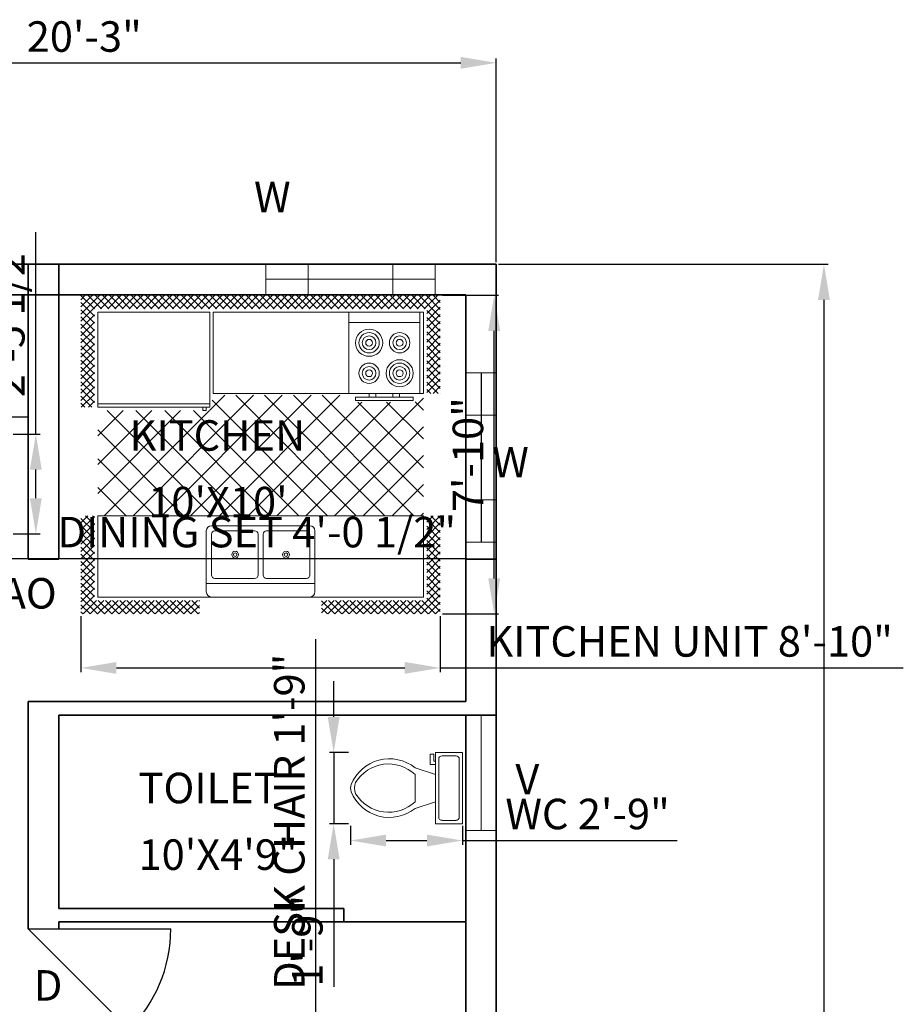
# Model space of a CAD drawing. Units: inches. Extents: x 1956 to 4770, y 1551 to 2596.
# Tile 7 of 10: x 2361 to 2621, y 2091 to 2381. Entities that reach past the tile are written whole.
import ezdxf

# ---------------------------------------------------------------- set-up
doc = ezdxf.new("R2010")
doc.units = ezdxf.units.IN
for name, color, linetype, lineweight in [('A-ANNO-DIMS', 2, 'Continuous', 18), ('A-ANNO-TEXT', 7, 'Continuous', 18), ('A-AREA-IDEN', 7, 'Continuous', 18), ('A-DOOR', 3, 'Continuous', 25), ('A-FLOR-FIXT', 9, 'Continuous', 18), ('A-FLOR-STRS', 7, 'Continuous', 25), ('A-GLAZ', 4, 'Continuous', 18), ('A-WALL', 7, 'Continuous', 35)]:
    doc.layers.add(name, color=color, linetype=linetype, lineweight=lineweight)
doc.styles.get("Standard").update_dxf_attribs({"font": 'arial.ttf'})
doc.dimstyles.new('ISO-25', dxfattribs={"dimtxt": 9, "dimasz": 10.5, "dimexe": 1.25, "dimexo": 0.625, "dimgap": 2, "dimtad": 1, "dimdec": 1, "dimlunit": 4, "dimtxsty": 'Standard', "dimcen": 2.5, "dimadec": 0, "dimazin": 0, "dimtfac": 1, "dimtdec": 1, "dimtmove": 0, "dimatfit": 3, "dimfxl": 1, "dimarcsym": 0})

# ---------------------------------------------------------------- blocks, each defined once
blk = doc.blocks.new('*D1')
at = {"layer": 'A-ANNO-DIMS', "color": 0, "lineweight": -2, "transparency": 16777216}
for p, q in [((2501.88, 2309.09), (2599.11, 2309.09)), ((2597.86, 2298.59), (2597.86, 1767.59)), ((2501.88, 1757.09), (2599.11, 1757.09))]:
    blk.add_line(p, q, dxfattribs=at)
at = {"layer": 'A-ANNO-DIMS', "color": 0, "transparency": 16777216}
for points in [[(2596.11, 2298.59), (2599.61, 2298.59), (2597.86, 2309.09)], [(2596.11, 1767.59), (2599.61, 1767.59), (2597.86, 1757.09)]]:
    blk.add_solid(points, dxfattribs=at)
at = {"layer": 'Defpoints', "color": 0, "transparency": 16777216}
for p in [(2501.25, 2309.09), (2501.25, 1757.09), (2597.86, 1757.09)]:
    blk.add_point(p, dxfattribs=at)
at = {"layer": 'A-ANNO-DIMS', "color": 0, "transparency": 16777216, "insert": (2591.27, 2033.09), "char_height": 9, "attachment_point": 5, "rotation": 90}
blk.add_mtext("46'", dxfattribs=at)
blk = doc.blocks.new('*D2')
at = {"layer": 'A-ANNO-DIMS', "color": 0, "lineweight": -2, "transparency": 16777216}
for p, q in [((2258.25, 2309.71), (2258.25, 2369.74)), ((2268.75, 2368.49), (2490.75, 2368.49)), ((2501.25, 2309.71), (2501.25, 2369.74))]:
    blk.add_line(p, q, dxfattribs=at)
at = {"layer": 'A-ANNO-DIMS', "color": 0, "transparency": 16777216}
for points in [[(2268.75, 2370.24), (2268.75, 2366.74), (2258.25, 2368.49)], [(2490.75, 2370.24), (2490.75, 2366.74), (2501.25, 2368.49)]]:
    blk.add_solid(points, dxfattribs=at)
at = {"layer": 'Defpoints', "color": 0, "transparency": 16777216}
for p in [(2501.25, 2368.49), (2258.25, 2309.09), (2501.25, 2309.09)]:
    blk.add_point(p, dxfattribs=at)
at = {"layer": 'A-ANNO-DIMS', "color": 0, "transparency": 16777216, "insert": (2379.75, 2375.08), "char_height": 9, "attachment_point": 5}
blk.add_mtext('20\'-3"', dxfattribs=at)
blk = doc.blocks.new('Kitchen Layout - 7 x 8 ft')
for p, q in [((-5, 81.32), (2.68, 89)), ((-5, 83.44), (0.56, 89)), ((-5, 85.56), (-1.56, 89)), ((-5, 87.68), (-3.68, 89)), ((-1, 84.97), (-5, 88.97)), ((1.09, 85), (-2.91, 89)), ((3.21, 85), (-0.79, 89)), ((0.81, 85), (4.81, 89)), ((5.34, 85), (1.34, 89)), ((2.93, 85), (6.93, 89)), ((7.46, 85), (3.46, 89)), ((5.05, 85), (9.05, 89)), ((9.58, 85), (5.58, 89)), ((7.17, 85), (11.17, 89)), ((11.7, 85), (7.7, 89)), ((9.29, 85), (13.29, 89)), ((13.82, 85), (9.82, 89)), ((11.41, 85), (15.41, 89)), ((15.94, 85), (11.94, 89)), ((13.53, 85), (17.53, 89)), ((18.06, 85), (14.06, 89)), ((15.65, 85), (19.65, 89)), ((20.18, 85), (16.18, 89)), ((17.78, 85), (21.78, 89)), ((22.31, 85), (18.31, 89)), ((19.9, 85), (23.9, 89)), ((24.43, 85), (20.43, 89)), ((22.02, 85), (26.02, 89)), ((26.55, 85), (22.55, 89)), ((24.14, 85), (28.14, 89)), ((28.67, 85), (24.67, 89)), ((26.26, 85), (30.26, 89)), ((30.79, 85), (26.79, 89)), ((28.38, 85), (32.38, 89)), ((32.91, 85), (28.91, 89)), ((30.5, 85), (34.5, 89)), ((35.03, 85), (31.03, 89)), ((32.63, 85), (36.63, 89)), ((37.16, 85), (33.16, 89)), ((34.75, 85), (38.75, 89)), ((39.28, 85), (35.28, 89)), ((36.87, 85), (40.87, 89)), ((41.4, 85), (37.4, 89)), ((38.99, 85), (42.99, 89)), ((43.52, 85), (39.52, 89)), ((41.11, 85), (45.11, 89)), ((45.64, 85), (41.64, 89)), ((43.23, 85), (47.23, 89)), ((47.76, 85), (43.76, 89)), ((45.35, 85), (49.35, 89)), ((49.88, 85), (45.88, 89)), ((47.47, 85), (51.47, 89)), ((52, 85), (48, 89)), ((49.6, 85), (53.6, 89)), ((54.13, 85), (50.13, 89)), ((51.72, 85), (55.72, 89)), ((56.25, 85), (52.25, 89)), ((53.84, 85), (57.84, 89)), ((58.37, 85), (54.37, 89)), ((55.96, 85), (59.96, 89)), ((60.49, 85), (56.49, 89)), ((58.08, 85), (62.08, 89)), ((62.61, 85), (58.61, 89)), ((60.2, 85), (64.2, 89)), ((64.73, 85), (60.73, 89)), ((62.32, 85), (66.32, 89)), ((66.85, 85), (62.85, 89)), ((64.45, 85), (68.45, 89)), ((68.97, 85), (64.97, 89)), ((66.57, 85), (70.57, 89)), ((71.1, 85), (67.1, 89)), ((68.69, 85), (72.69, 89)), ((73.22, 85), (69.22, 89)), ((70.81, 85), (74.81, 89)), ((75.34, 85), (71.34, 89)), ((72.93, 85), (76.93, 89)), ((77.46, 85), (73.46, 89)), ((75.05, 85), (79.05, 89)), ((79.58, 85), (75.58, 89)), ((77.17, 85), (81.17, 89)), ((81.7, 85), (77.7, 89)), ((79.29, 85), (83.29, 89)), ((83.82, 85), (79.82, 89)), ((81.42, 85), (85.42, 89)), ((85.95, 85), (81.95, 89)), ((83.54, 85), (87.54, 89)), ((88.07, 85), (84.07, 89)), ((85.66, 85), (89.66, 89)), ((90.19, 85), (86.19, 89)), ((87.78, 85), (91.78, 89)), ((92.31, 85), (88.31, 89)), ((89.9, 85), (93.9, 89)), ((94.43, 85), (90.43, 89)), ((92.02, 85), (96.02, 89)), ((96.55, 85), (92.55, 89)), ((94.14, 85), (98.14, 89)), ((101, 82.67), (94.67, 89)), ((96.27, 85), (100.27, 89)), ((101, 84.79), (96.79, 89)), ((97, 83.61), (101, 87.61)), ((101, 86.92), (98.92, 89)), ((-1, 82.85), (-5, 86.85)), ((-1, 80.73), (-5, 84.73)), ((97, 81.49), (101, 85.49)), ((101, 80.55), (97, 84.55)), ((-5, 79.19), (-1, 83.19)), ((-1, 78.61), (-5, 82.61)), ((34, 84), (96, 84)), ((34, 60), (34, 84)), ((96, 84), (96, 60)), ((97, 79.37), (101, 83.37)), ((101, 78.43), (97, 82.43)), ((-5, 77.07), (-1, 81.07)), ((-1, 76.49), (-5, 80.49)), ((-5, 74.95), (-1, 78.95)), ((74, 81), (95, 81)), ((97, 77.25), (101, 81.25)), ((101, 76.31), (97, 80.31)), ((97, 75.13), (101, 79.13)), ((-1, 74.36), (-5, 78.36)), ((-5, 72.83), (-1, 76.83)), ((-1, 72.24), (-5, 76.24)), ((101, 74.19), (97, 78.19)), ((97, 73.01), (101, 77.01)), ((101, 72.07), (97, 76.07)), ((-5, 70.71), (-1, 74.71)), ((-1, 70.12), (-5, 74.12)), ((97, 70.89), (101, 74.89)), ((101, 69.95), (97, 73.95)), ((97, 68.76), (101, 72.76)), ((-5, 68.59), (-1, 72.59)), ((-1, 68), (-5, 72)), ((-5, 66.47), (-1, 70.47)), ((-1, 65.88), (-5, 69.88)), ((101, 67.82), (97, 71.82)), ((97, 66.64), (101, 70.64)), ((101, 65.7), (97, 69.7)), ((-5, 64.35), (-1, 68.35)), ((-1, 63.76), (-5, 67.76)), ((97, 64.52), (101, 68.52)), ((101, 63.58), (97, 67.58)), ((-5, 62.22), (-1, 66.22)), ((-1, 61.64), (-5, 65.64)), ((-5, 60.1), (-1, 64.1)), ((97, 62.4), (101, 66.4)), ((101, 61.46), (97, 65.46)), ((97, 60.28), (101, 64.28)), ((-1, 59.52), (-5, 63.52)), ((-5, 57.98), (-1, 61.98)), ((-1, 57.39), (-5, 61.39)), ((100.34, 60), (97, 63.34)), ((98.22, 60), (97, 61.22)), ((98.84, 60), (101, 62.16)), ((-1.73, 56), (-5, 59.27)), ((-4.86, 56), (-1, 59.86)), ((10.4, 24), (45.9, 59.5)), ((18.88, 24), (54.38, 59.5)), ((27.37, 24), (62.87, 59.5)), ((33.03, 55.11), (37.41, 59.5)), ((96, 60), (34, 60)), ((35.85, 24), (71.35, 59.5)), ((76.2, 24), (40.7, 59.5)), ((84.68, 24), (49.18, 59.5)), ((93.17, 24), (57.67, 59.5)), ((61.31, 24), (96, 58.69)), ((96, 29.65), (66.15, 59.5)), ((80, 60), (80, 59)), ((82, 59), (82, 60)), ((87, 59), (87, 60)), ((89, 60), (89, 59)), ((100.96, 60), (101, 60.04)), ((-3.85, 56), (-5, 57.15)), ((-2.74, 56), (-1, 57.74)), ((0, 57), (33, 57)), ((31, 55), (31, 56)), ((32, 56), (32, 55)), ((67.71, 24), (33.68, 58.04)), ((44.34, 24), (77.84, 57.5)), ((52.82, 24), (86.32, 57.5)), ((96, 38.14), (76.64, 57.5)), ((96, 46.63), (85.13, 57.5)), ((96, 55.11), (93.57, 57.54)), ((0, 30.57), (24.43, 55)), ((0, 39.06), (15.94, 55)), ((0, 47.54), (7.46, 55)), ((1.91, 24), (32.91, 55)), ((33.77, 24), (2.77, 55)), ((42.26, 24), (11.26, 55)), ((50.74, 24), (19.74, 55)), ((59.23, 24), (28.23, 55)), ((32, 55), (31, 55)), ((69.79, 24), (96, 50.21)), ((25.29, 24), (0, 49.29)), ((16.8, 24), (0, 40.8)), ((78.28, 24), (96, 41.72)), ((8.32, 24), (0, 32.32)), ((86.76, 24), (96, 33.24)), ((-5, 21.92), (-2.92, 24)), ((-5, 19.8), (-1, 23.8)), ((-1, 21.33), (-3.67, 24)), ((-1, 23.45), (-1.55, 24)), ((0, 24), (96, 24)), ((0, 0), (0, 24)), ((95.25, 24), (96, 24.75)), ((96, 24), (96, 0)), ((97, 22.1), (98.9, 24)), ((97, 19.97), (101, 23.97)), ((101, 21.16), (98.16, 24)), ((101, 23.28), (100.28, 24)), ((-1, 19.21), (-5, 23.21)), ((-5, 17.68), (-1, 21.68)), ((-1, 17.09), (-5, 21.09)), ((101, 19.03), (97, 23.03)), ((97, 17.85), (101, 21.85)), ((101, 16.91), (97, 20.91)), ((-5, 15.55), (-1, 19.55)), ((-1, 14.97), (-5, 18.97)), ((-5, 13.43), (-1, 17.43)), ((47.25, 6.5), (47.25, 18.5)), ((48.75, 18.5), (48.75, 6.5)), ((97, 15.73), (101, 19.73)), ((101, 14.79), (97, 18.79)), ((97, 13.61), (101, 17.61)), ((-1, 12.85), (-5, 16.85)), ((-5, 11.31), (-1, 15.31)), ((-1, 10.73), (-5, 14.73)), ((101, 12.67), (97, 16.67)), ((97, 11.49), (101, 15.49)), ((101, 10.55), (97, 14.55)), ((-5, 9.19), (-1, 13.19)), ((-1, 8.6), (-5, 12.6)), ((97, 9.37), (101, 13.37)), ((101, 8.43), (97, 12.43)), ((-5, 7.07), (-1, 11.07)), ((-1, 6.48), (-5, 10.48)), ((-5, 4.95), (-1, 8.95)), ((97, 7.25), (101, 11.25)), ((101, 6.31), (97, 10.31)), ((97, 5.12), (101, 9.12)), ((-1, 4.36), (-5, 8.36)), ((-5, 2.83), (-1, 6.83)), ((-1, 2.24), (-5, 6.24)), ((101, 4.18), (97, 8.18)), ((97, 3), (101, 7)), ((101, 2.06), (97, 6.06)), ((-5, 0.71), (-1, 4.71)), ((-1, 0.12), (-5, 4.12)), ((64, 4), (32, 4)), ((97, 0.88), (101, 4.88)), ((101, -0.06), (97, 3.94)), ((-5, -1.42), (-1, 2.58)), ((2, -5), (-5, 2)), ((-5, -3.54), (-1, 0.46)), ((96, 0), (0, 0)), ((93.24, -5), (101, 2.76)), ((95.36, -5), (101, 0.64)), ((101, -2.18), (97, 1.82)), ((-0.12, -5), (-5, -0.12)), ((-2.25, -5), (-5, -2.25)), ((-4.34, -5), (-0.34, -1)), ((-2.22, -5), (1.78, -1)), ((-0.1, -5), (3.9, -1)), ((4.12, -5), (0.12, -1)), ((2.02, -5), (6.02, -1)), ((6.24, -5), (2.24, -1)), ((4.14, -5), (8.14, -1)), ((8.36, -5), (4.36, -1)), ((6.27, -5), (10.27, -1)), ((10.48, -5), (6.48, -1)), ((8.39, -5), (12.39, -1)), ((12.6, -5), (8.6, -1)), ((10.51, -5), (14.51, -1)), ((14.73, -5), (10.73, -1)), ((12.63, -5), (16.63, -1)), ((16.85, -5), (12.85, -1)), ((14.75, -5), (18.75, -1)), ((18.97, -5), (14.97, -1)), ((16.87, -5), (20.87, -1)), ((21.09, -5), (17.09, -1)), ((18.99, -5), (22.99, -1)), ((23.21, -5), (19.21, -1)), ((21.11, -5), (25.11, -1)), ((25.33, -5), (21.33, -1)), ((23.24, -5), (27.24, -1)), ((27.45, -5), (23.45, -1)), ((25.36, -5), (29.36, -1)), ((29.57, -5), (25.57, -1)), ((27.48, -5), (30, -2.48)), ((30, -3.3), (27.7, -1)), ((30, -1.18), (29.82, -1)), ((66, -2.54), (67.54, -1)), ((66, -4.66), (69.66, -1)), ((69.88, -5), (66, -1.12)), ((67.78, -5), (71.78, -1)), ((72, -5), (68, -1)), ((69.9, -5), (73.9, -1)), ((74.12, -5), (70.12, -1)), ((72.03, -5), (76.03, -1)), ((76.24, -5), (72.24, -1)), ((74.15, -5), (78.15, -1)), ((78.36, -5), (74.36, -1)), ((76.27, -5), (80.27, -1)), ((80.49, -5), (76.49, -1)), ((78.39, -5), (82.39, -1)), ((82.61, -5), (78.61, -1)), ((80.51, -5), (84.51, -1)), ((84.73, -5), (80.73, -1)), ((82.63, -5), (86.63, -1)), ((86.85, -5), (82.85, -1)), ((84.75, -5), (88.75, -1)), ((88.97, -5), (84.97, -1)), ((86.88, -5), (90.88, -1)), ((91.09, -5), (87.09, -1)), ((89, -5), (93, -1)), ((93.21, -5), (89.21, -1)), ((91.12, -5), (95.12, -1)), ((95.34, -5), (91.34, -1)), ((97.46, -5), (93.46, -1)), ((99.58, -5), (95.58, -1)), ((101, -4.3), (97, -0.3)), ((97.48, -5), (101, -1.48)), ((-4.37, -5), (-5, -4.37)), ((29.6, -5), (30, -4.6)), ((67.76, -5), (66, -3.24)), ((99.6, -5), (101, -3.6))]:
    blk.add_line(p, q)
for points in [[(0, 56), (0, 84), (33, 84), (33, 56)], [(74, 60), (74, 84), (95, 84), (95, 60)], [(76, 58), (76, 59), (93, 59), (93, 58)]]:
    blk.add_lwpolyline(points, close=True)
for points in [[(33.5, 21), (62.5, 21)], [(32, 1.5), (32, 19.5)], [(33.5, 6.5), (33.5, 18.5)], [(34.5, 19.5), (46.25, 19.5)], [(49.75, 19.5), (61.5, 19.5)], [(62.5, 18.5), (62.5, 6.5)], [(64, 19.5), (64, 1.5)], [(46.25, 5.5), (34.5, 5.5)], [(61.5, 5.5), (49.75, 5.5)], [(62.5, 0), (33.5, 0)]]:
    blk.add_lwpolyline(points)
for centre, radius in [((80, 75), 4), ((80, 75), 3), ((80, 75), 2), ((80, 75), 1), ((89, 75), 3), ((89, 75), 2), ((89, 75), 1), ((89, 66), 4), ((80, 66), 3), ((80, 66), 2), ((80, 66), 1), ((89, 66), 3), ((89, 66), 2), ((89, 66), 1), ((40.5, 12.5), 1), ((40.5, 12.5), 0.5), ((55.5, 12.5), 1), ((55.5, 12.5), 0.5)]:
    blk.add_circle(centre, radius)
for centre, radius, start, end in [((33.5, 19.5), 1.5, 90, 180), ((62.5, 19.5), 1.5, 0, 90), ((34.5, 18.5), 1, 90, 180), ((46.25, 18.5), 1, 0, 90), ((49.75, 18.5), 1, 90, 180), ((61.5, 18.5), 1, 0, 90), ((34.5, 6.5), 1, 180, 270), ((46.25, 6.5), 1, 270, 0), ((49.75, 6.5), 1, 180, 270), ((61.5, 6.5), 1, 270, 0), ((33.5, 1.5), 1.5, 180, 270), ((62.5, 1.5), 1.5, 270, 0)]:
    blk.add_arc(centre, radius, start, end)
blk = doc.blocks.new('Toilet - top')
for p, q in [((9.5, -6), (9.5, -2)), ((-10, -8.5), (-8, -8.5)), ((-10, -9.5), (-10, -8.5)), ((-8, -8.5), (-8, -8)), ((-7, -8), (-7, -9.5)), ((-4, -8), (-6, -14)), ((4, -8), (6, -14)), ((-7, -9.5), (-10, -9.5)), ((4, -14), (-4, -14))]:
    blk.add_line(p, q)
blk.add_lwpolyline([(10.5, -8), (10.5, 0), (-10.5, 0), (-10.5, -8)], close=True)
for points in [[(-9.5, -2), (-9.5, -6)], [(8.5, -1), (-8.5, -1)], [(-8.5, -7), (8.5, -7)]]:
    blk.add_lwpolyline(points)
for centre, radius, start, end in [((-8.62, -1.88), 0.884, 81.8699, 188.1301), ((8.62, -1.88), 0.884, 351.8699, 98.1301), ((-8.62, -6.12), 0.884, 171.8699, 278.1301), ((8.62, -6.12), 0.884, 261.8699, 8.1301), ((3.52, -21.58), 12.17, 141.4691, 247.9714), ((4.2, -21.82), 11.33, 136.3677, 238.9468), ((-3.52, -21.58), 12.17, 292.0284, 38.5307), ((-4.2, -21.82), 11.33, 301.053, 43.6321), ((0, -27.88), 4, 245.7318, 294.2682), ((0, -29), 4, 254.8605, 285.1395)]:
    blk.add_arc(centre, radius, start, end)
blk = doc.blocks.new('WIN-50IN-WALL9')
for p, q in [((0, 50), (9, 50)), ((4.6, 50), (4.6, 0)), ((0, 37.5), (9, 37.5)), ((9, 12.5), (0, 12.5)), ((9, 0), (1, 0)), ((0, 0), (9, 0))]:
    blk.add_line(p, q)
blk = doc.blocks.new('*D43')
at = {"layer": 'A-ANNO-DIMS', "color": 0, "lineweight": -2, "transparency": 16777216}
for p, q in [((2378.74, 2205.3), (2378.74, 2188.78)), ((2484.74, 2205.3), (2484.74, 2188.78)), ((2389.24, 2190.03), (2474.24, 2190.03)), ((2484.74, 2190.03), (2621.26, 2190.03))]:
    blk.add_line(p, q, dxfattribs=at)
at = {"layer": 'A-ANNO-DIMS', "color": 0, "transparency": 16777216}
for points in [[(2389.24, 2191.78), (2389.24, 2188.28), (2378.74, 2190.03)], [(2474.24, 2191.78), (2474.24, 2188.28), (2484.74, 2190.03)]]:
    blk.add_solid(points, dxfattribs=at)
at = {"layer": 'Defpoints', "color": 0, "transparency": 16777216}
for p in [(2378.74, 2205.93), (2484.74, 2205.93), (2484.74, 2190.03)]:
    blk.add_point(p, dxfattribs=at)
at = {"layer": 'A-ANNO-DIMS', "color": 0, "transparency": 16777216, "insert": (2558.25, 2196.68), "char_height": 9, "attachment_point": 5}
blk.add_mtext('KITCHEN UNIT 8\'-10"', dxfattribs=at)
blk = doc.blocks.new('*D44')
at = {"layer": 'A-ANNO-DIMS', "color": 0, "lineweight": -2, "transparency": 16777216}
for p, q in [((2485.36, 2299.93), (2501.89, 2299.93)), ((2500.64, 2216.43), (2500.64, 2289.43)), ((2485.36, 2205.93), (2501.89, 2205.93))]:
    blk.add_line(p, q, dxfattribs=at)
at = {"layer": 'A-ANNO-DIMS', "color": 0, "transparency": 16777216}
for points in [[(2498.89, 2289.43), (2502.39, 2289.43), (2500.64, 2299.93)], [(2498.89, 2216.43), (2502.39, 2216.43), (2500.64, 2205.93)]]:
    blk.add_solid(points, dxfattribs=at)
at = {"layer": 'Defpoints', "color": 0, "transparency": 16777216}
for p in [(2484.74, 2299.93), (2500.64, 2299.93), (2484.74, 2205.93)]:
    blk.add_point(p, dxfattribs=at)
at = {"layer": 'A-ANNO-DIMS', "color": 0, "transparency": 16777216, "insert": (2494.04, 2252.93), "char_height": 9, "attachment_point": 5, "rotation": 90}
blk.add_mtext('7\'-10"', dxfattribs=at)
blk = doc.blocks.new('*D49')
at = {"layer": 'A-ANNO-DIMS', "color": 0, "lineweight": -2, "transparency": 16777216}
for p, q in [((2458.25, 2143.45), (2458.25, 2137.86)), ((2491.29, 2143.45), (2491.29, 2137.86)), ((2468.75, 2139.11), (2480.79, 2139.11)), ((2491.29, 2139.11), (2554.53, 2139.11))]:
    blk.add_line(p, q, dxfattribs=at)
at = {"layer": 'A-ANNO-DIMS', "color": 0, "transparency": 16777216}
for points in [[(2468.75, 2140.86), (2468.75, 2137.36), (2458.25, 2139.11)], [(2480.79, 2140.86), (2480.79, 2137.36), (2491.29, 2139.11)]]:
    blk.add_solid(points, dxfattribs=at)
at = {"layer": 'Defpoints', "color": 0, "transparency": 16777216}
for p in [(2458.25, 2144.07), (2491.29, 2144.07), (2491.29, 2139.11)]:
    blk.add_point(p, dxfattribs=at)
at = {"layer": 'A-ANNO-DIMS', "color": 0, "transparency": 16777216, "insert": (2528.16, 2145.77), "char_height": 9, "attachment_point": 5}
blk.add_mtext('WC 2\'-9"', dxfattribs=at)
blk = doc.blocks.new('*D50')
at = {"layer": 'A-ANNO-DIMS', "color": 0, "lineweight": -2, "transparency": 16777216}
for p, q in [((2453.29, 2175.57), (2453.29, 2186.07)), ((2457.62, 2165.07), (2452.04, 2165.07)), ((2453.29, 2165.07), (2453.29, 2144.07)), ((2457.62, 2144.07), (2452.04, 2144.07)), ((2453.29, 2133.57), (2453.29, 2095.99))]:
    blk.add_line(p, q, dxfattribs=at)
at = {"layer": 'A-ANNO-DIMS', "color": 0, "transparency": 16777216}
for points in [[(2451.54, 2175.57), (2455.04, 2175.57), (2453.29, 2165.07)], [(2451.54, 2133.57), (2455.04, 2133.57), (2453.29, 2144.07)]]:
    blk.add_solid(points, dxfattribs=at)
at = {"layer": 'Defpoints', "color": 0, "transparency": 16777216}
for p in [(2458.25, 2165.07), (2453.29, 2144.07), (2458.25, 2144.07)]:
    blk.add_point(p, dxfattribs=at)
at = {"layer": 'A-ANNO-DIMS', "color": 0, "transparency": 16777216, "insert": (2446.7, 2109.53), "char_height": 9, "attachment_point": 5, "rotation": 90}
blk.add_mtext('1\'-9"', dxfattribs=at)
blk = doc.blocks.new('*D51')
at = {"layer": 'A-ANNO-DIMS', "color": 0, "lineweight": -2, "transparency": 16777216}
for p, q in [((2309.47, 2228.95), (2309.47, 2221.02)), ((2358.16, 2228.95), (2358.16, 2221.02)), ((2319.97, 2222.27), (2347.66, 2222.27)), ((2358.16, 2222.27), (2492.55, 2222.27))]:
    blk.add_line(p, q, dxfattribs=at)
at = {"layer": 'A-ANNO-DIMS', "color": 0, "transparency": 16777216}
for points in [[(2319.97, 2224.02), (2319.97, 2220.52), (2309.47, 2222.27)], [(2347.66, 2224.02), (2347.66, 2220.52), (2358.16, 2222.27)]]:
    blk.add_solid(points, dxfattribs=at)
at = {"layer": 'Defpoints', "color": 0, "transparency": 16777216}
for p in [(2309.47, 2229.57), (2358.16, 2229.57), (2358.16, 2222.27)]:
    blk.add_point(p, dxfattribs=at)
at = {"layer": 'A-ANNO-DIMS', "color": 0, "transparency": 16777216, "insert": (2430.61, 2228.92), "char_height": 9, "attachment_point": 5}
blk.add_mtext('DINING SET 4\'-0 1/2"', dxfattribs=at)
blk = doc.blocks.new('*D52')
at = {"layer": 'A-ANNO-DIMS', "color": 0, "lineweight": -2, "transparency": 16777216}
for p, q in [((2365.47, 2259), (2365.47, 2318.55)), ((2358.79, 2259), (2366.72, 2259)), ((2365.47, 2240.07), (2365.47, 2248.5)), ((2358.79, 2229.57), (2366.72, 2229.57))]:
    blk.add_line(p, q, dxfattribs=at)
at = {"layer": 'A-ANNO-DIMS', "color": 0, "transparency": 16777216}
for points in [[(2363.72, 2248.5), (2367.22, 2248.5), (2365.47, 2259)], [(2363.72, 2240.07), (2367.22, 2240.07), (2365.47, 2229.57)]]:
    blk.add_solid(points, dxfattribs=at)
at = {"layer": 'Defpoints', "color": 0, "transparency": 16777216}
for p in [(2358.16, 2259), (2365.47, 2259), (2358.16, 2229.57)]:
    blk.add_point(p, dxfattribs=at)
at = {"layer": 'A-ANNO-DIMS', "color": 0, "transparency": 16777216, "insert": (2358.81, 2294.03), "char_height": 9, "attachment_point": 5, "rotation": 90}
blk.add_mtext('2\'-5 1/2"', dxfattribs=at)
blk = doc.blocks.new('*D57')
at = {"layer": 'A-ANNO-DIMS', "color": 0, "lineweight": -2, "transparency": 16777216}
for p, q in [((2448.01, 2080.23), (2448.01, 2198.55)), ((2450.54, 2069.73), (2446.76, 2069.73)), ((2448.01, 2048.73), (2448.01, 2069.73)), ((2450.54, 2048.73), (2446.76, 2048.73)), ((2448.01, 2038.23), (2448.01, 2027.73))]:
    blk.add_line(p, q, dxfattribs=at)
at = {"layer": 'A-ANNO-DIMS', "color": 0, "transparency": 16777216}
for points in [[(2446.26, 2080.23), (2449.76, 2080.23), (2448.01, 2069.73)], [(2446.26, 2038.23), (2449.76, 2038.23), (2448.01, 2048.73)]]:
    blk.add_solid(points, dxfattribs=at)
at = {"layer": 'Defpoints', "color": 0, "transparency": 16777216}
for p in [(2448.01, 2069.73), (2451.16, 2069.73), (2451.16, 2048.73)]:
    blk.add_point(p, dxfattribs=at)
at = {"layer": 'A-ANNO-DIMS', "color": 0, "transparency": 16777216, "insert": (2441.36, 2144.64), "char_height": 9, "attachment_point": 5, "rotation": 90}
blk.add_mtext('DESK CHAIR 1\'-9"', dxfattribs=at)
blk = doc.blocks.new('*D105')
at = {"layer": 'A-ANNO-DIMS', "color": 0, "lineweight": -2, "transparency": 16777216}
for p, q in [((2363.25, 2113.09), (2392.95, 2083.39)), ((2433.64, 2042.7), (2400.38, 2075.96))]:
    blk.add_line(p, q, dxfattribs=at)
at = {"layer": 'A-ANNO-DIMS', "color": 0, "transparency": 16777216}
blk.add_solid([(2401.61, 2077.2), (2399.14, 2074.73), (2392.95, 2083.39)], dxfattribs=at)
at = {"layer": 'Defpoints', "color": 0, "transparency": 16777216}
for p in [(2363.25, 2113.09), (2392.95, 2083.39)]:
    blk.add_point(p, dxfattribs=at)
at = {"layer": 'A-ANNO-DIMS', "color": 0, "transparency": 16777216, "insert": (2425.39, 2060.29), "char_height": 9, "attachment_point": 5, "rotation": 315.0003}
blk.add_mtext('R3\'-6"', dxfattribs=at)

msp = doc.modelspace()

# ---------------------------------------------------------------- linework, layer by layer
at = {"layer": 'A-DOOR'}
msp.add_line((2363.25, 2113.09), (2405.25, 2113.09), dxfattribs=at)
msp.add_arc((2363.25, 2113.09), 42, 270, 0, dxfattribs=at)
at = {"layer": 'A-FLOR-STRS'}
msp.add_line((2303.25, 2264.09), (2363.25, 2264.09), dxfattribs=at)
at = {"layer": 'A-GLAZ'}
for p, q in [((2483.25, 2309.09), (2483.25, 2301.09)), ((2492.25, 2277.09), (2501.25, 2277.09)), ((2492.25, 2277.09), (2501.25, 2277.09)), ((2496.75, 2277.09), (2496.75, 2227.09)), ((2496.75, 2252.09), (2496.85, 2252.09)), ((2492.25, 2227.09), (2501.25, 2227.09)), ((2492.25, 2227.09), (2501.25, 2227.09)), ((2492.25, 2176.09), (2501.25, 2176.09)), ((2496.75, 2176.09), (2496.75, 2142.09)), ((2492.25, 2142.09), (2501.25, 2142.09))]:
    msp.add_line(p, q, dxfattribs=at)
at = {"layer": 'A-WALL'}
for p, q in [((2258.25, 2309.09), (2501.25, 2309.09)), ((2363.25, 2222.09), (2363.25, 2309.09)), ((2372.25, 2222.09), (2372.25, 2309.09)), ((2501.25, 2309.09), (2501.25, 1909.09)), ((2258.25, 2300.09), (2492.25, 2300.09)), ((2492.25, 2300.09), (2492.25, 2180.09)), ((2363.25, 2222.09), (2372.25, 2222.09)), ((2492.25, 2222.09), (2501.25, 2222.09)), ((2363.25, 2180.09), (2492.25, 2180.09)), ((2363.25, 2113.09), (2363.25, 2180.09)), ((2372.25, 2176.09), (2501.25, 2176.09)), ((2372.25, 2119.09), (2372.25, 2176.09)), ((2492.25, 2176.09), (2492.25, 1910.09)), ((2372.25, 2119.09), (2456.25, 2119.09)), ((2456.25, 2119.09), (2456.25, 2115.09)), ((2372.25, 2115.09), (2492.25, 2115.09)), ((2372.25, 2113.09), (2372.25, 2115.09)), ((2372.25, 2113.09), (2372.25, 2115.09))]:
    msp.add_line(p, q, dxfattribs=at)

# ---------------------------------------------------------------- block references
at = {"layer": 'A-FLOR-FIXT'}
msp.add_blockref('Kitchen Layout - 7 x 8 ft', (2383.74, 2210.93), dxfattribs=at)
at = {"layer": 'A-FLOR-FIXT', "rotation": 270}
msp.add_blockref('Toilet - top', (2491.29, 2154.57), dxfattribs=at)
at = {"layer": 'A-GLAZ', "rotation": 89.9999999999992}
msp.add_blockref('WIN-50IN-WALL9', (2483.25, 2300.09), dxfattribs=at)
at = {"layer": 'A-GLAZ'}
msp.add_blockref('WIN-50IN-WALL9', (2492.25, 2227.09), dxfattribs=at)

# ---------------------------------------------------------------- texts
at = {"layer": 'A-ANNO-TEXT'}
for s, p in [('  W', (2424.31, 2324.4)), ('         W ', (2475.32, 2246.23)), ('        AO', (2333.05, 2207.53)), ('         V ', (2482.1, 2152.71)), ('D', (2364.86, 2091.88))]:
    msp.add_text(s, height=9, dxfattribs=at).set_placement(p)
at = {"layer": 'A-AREA-IDEN'}
for s, p in [('KITCHEN', (2393.11, 2254.08)), ("  10'X10'", (2393.11, 2234.43)), ('TOILET', (2395.75, 2150.11)), ('10\'X4\'9"', (2395.75, 2130.46))]:
    msp.add_text(s, height=9, dxfattribs=at).set_placement(p)

# ---------------------------------------------------------------- dimensions: what is measured, and where the dimension line sits
at = {"layer": 'A-ANNO-DIMS'}
dim = msp.add_linear_dim(base=(2501.25, 2368.49), p1=(2258.25, 2309.09), p2=(2501.25, 2309.09), dimstyle='ISO-25', override={"dimclrd": 0, "dimclre": 0, "dimclrt": 0}, dxfattribs=at)
dim.commit()
dim.dimension.update_dxf_attribs({"geometry": '*D2', "text_midpoint": (2379.75, 2375.08)})
for base, p1, p2, angle, override, picture, middle in [((2365.47, 2259), (2358.16, 2229.57), (2358.16, 2259), 90, {"dimdec": 1, "dimlfac": 1, "dimrnd": 0, "dimzin": 1, "dimdsep": 46, "dimlunit": 4, "dimfrac": 2}, '*D52', (2358.81, 2294.03)), ((2597.86, 1757.09), (2501.25, 2309.09), (2501.25, 1757.09), 90, {"dimclrd": 0, "dimclre": 0, "dimclrt": 0}, '*D1', (2591.27, 2033.09)), ((2500.64, 2299.93), (2484.74, 2205.93), (2484.74, 2299.93), 90, {"dimdec": 1, "dimlfac": 1, "dimrnd": 0, "dimzin": 1, "dimdsep": 46, "dimlunit": 4, "dimfrac": 2}, '*D44', (2494.04, 2252.93)), ((2453.29, 2144.07), (2458.25, 2165.07), (2458.25, 2144.07), 270, {"dimdec": 1, "dimlfac": 1, "dimrnd": 0, "dimzin": 1, "dimdsep": 46, "dimlunit": 4, "dimfrac": 2}, '*D50', (2446.7, 2109.53))]:
    dim = msp.add_linear_dim(base=base, p1=p1, p2=p2, angle=angle, dimstyle='ISO-25', override=override, dxfattribs=at)
    dim.commit()
    dim.dimension.update_dxf_attribs({"geometry": picture, "text_midpoint": middle})
for base, p1, p2, text, picture, middle in [((2358.16, 2222.27), (2309.47, 2229.57), (2358.16, 2229.57), 'DINING SET <>', '*D51', (2430.61, 2228.92)), ((2484.74, 2190.03), (2378.74, 2205.93), (2484.74, 2205.93), 'KITCHEN UNIT <>', '*D43', (2558.25, 2196.68)), ((2491.29, 2139.11), (2458.25, 2144.07), (2491.29, 2144.07), 'WC <>', '*D49', (2528.16, 2145.77))]:
    dim = msp.add_linear_dim(base=base, p1=p1, p2=p2, text=text, dimstyle='ISO-25', override={"dimdec": 1, "dimlfac": 1, "dimrnd": 0, "dimzin": 1, "dimdsep": 46, "dimlunit": 4, "dimfrac": 2}, dxfattribs=at)
    dim.commit()
    dim.dimension.update_dxf_attribs({"geometry": picture, "text_midpoint": middle})
dim = msp.add_linear_dim(base=(2448.01, 2069.73), p1=(2451.16, 2048.73), p2=(2451.16, 2069.73), angle=90, text='DESK CHAIR <>', dimstyle='ISO-25', override={"dimdec": 1, "dimlfac": 1, "dimrnd": 0, "dimzin": 1, "dimdsep": 46, "dimlunit": 4, "dimfrac": 2}, dxfattribs=at)
dim.commit()
dim.dimension.update_dxf_attribs({"geometry": '*D57', "text_midpoint": (2441.36, 2144.64)})
dim = msp.add_radius_dim(center=(2363.25, 2113.09), mpoint=(2392.95, 2083.39), dimstyle='ISO-25', override={"dimdec": 1, "dimlfac": 1, "dimrnd": 0, "dimzin": 1, "dimdsep": 46, "dimlunit": 4, "dimfrac": 2}, dxfattribs=at)
dim.commit()
dim.dimension.update_dxf_attribs({"geometry": '*D105', "text_midpoint": (2425.39, 2060.29)})

doc.saveas('drawing.dxf')
